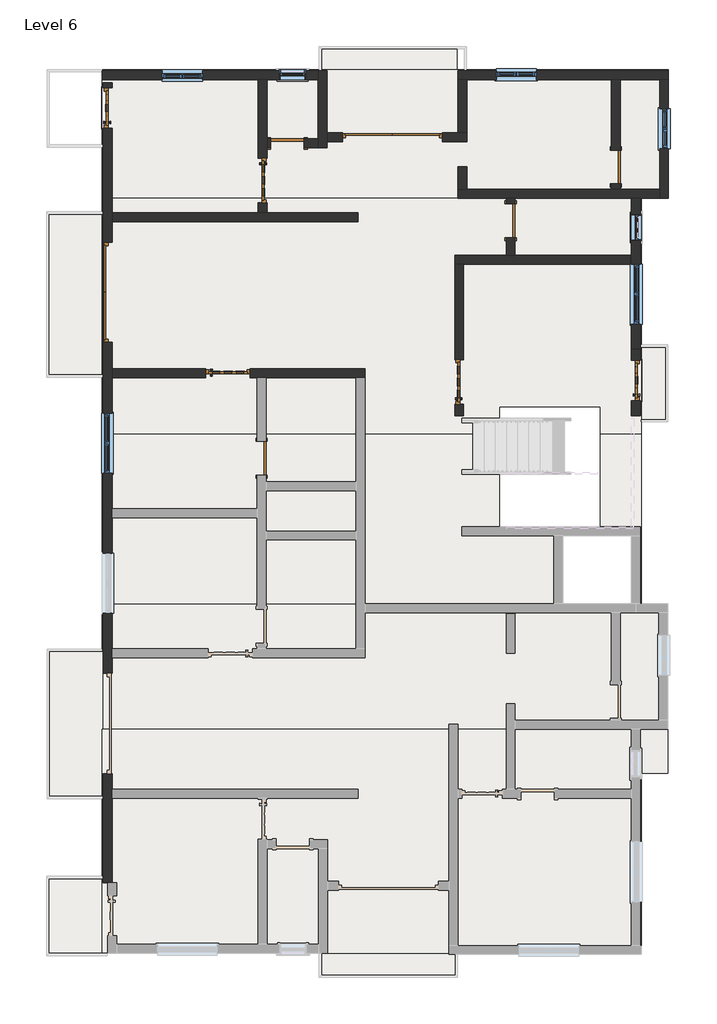
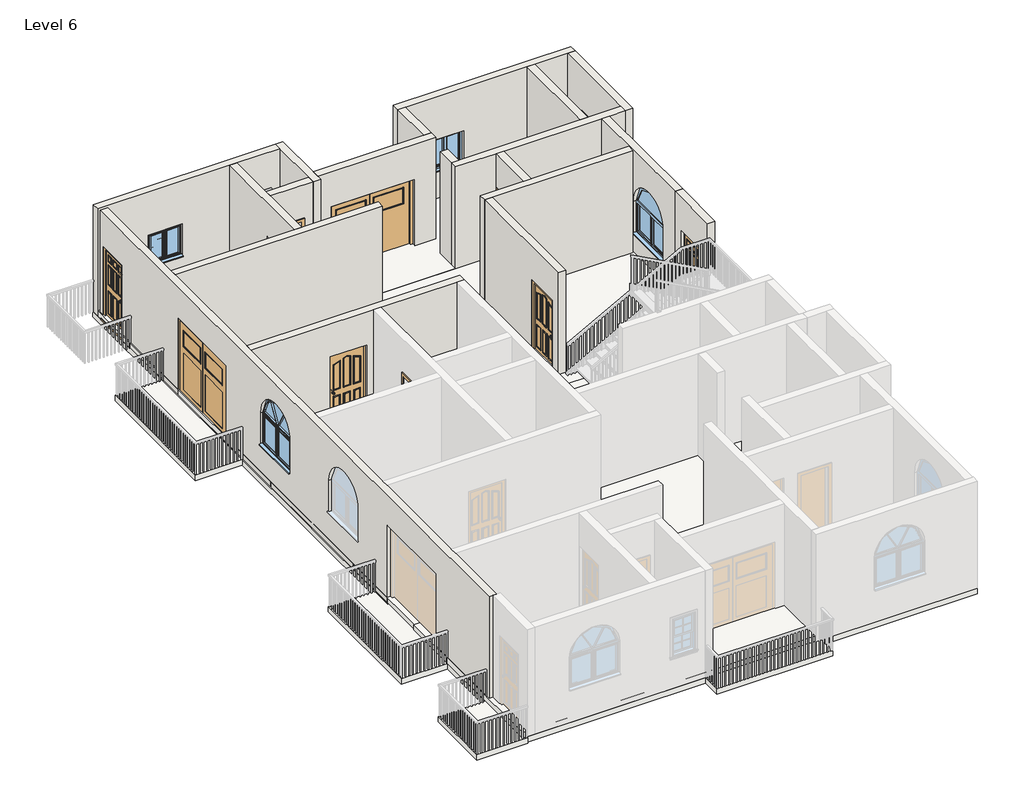
# One storey, part 2 of 7: 19 walls, 11 doors, 9 slabs, 7 windows, 5 roofs.
"""IFC4 building model written with IfcOpenShell, lengths in millimetres."""

from ifc_helpers import new_model, si_unit, point, frame, frame_2d, origin, place, context, project, spatial, polyline, circle_curve, trimmed, segment, composite_curve, outline, extrude, faceted_brep, transform, mapped, element, save
from ifc_brep_helpers import plane_surface, revolved_surface, advanced_brep
from components import doors_extsgl_5_910x2110mm_99758a98, doors_extsgl_5_910x2110mm_d3ca6061, doors_extsgl_6_1010x2110mm_b93c615f, doors_extsgl_6_1010x2110mm_efbaf1af, doors_garage_timber_side_hung_glazing_2270x2050mm_ae99176d, doors_garage_timber_side_hung_glazing_2270x2200mm_badb7014, door_53b1b562, window_679d2811, windows_arched_1360x910mm_c5754810, windows_dbl_w_glazing_bars_910x910mm_41eba874

model = new_model("IFC4")

# Units and contexts
model_context = context("Model", 3, world=origin())
ifc_project = project(units=[si_unit("LENGTHUNIT", "METRE", prefix="MILLI")], contexts=[model_context])

# Site, building, storey
site = spatial("IfcSite", under=ifc_project)
building = spatial("IfcBuilding", under=site)
storey = spatial("IfcBuildingStorey", under=building, Name="Level 6", Elevation=15240.0)

# Doors
placement = place(None, origin())
doors_extsgl_5_910x2110mm_shape = doors_extsgl_5_910x2110mm_99758a98(model_context)
element("IfcDoor", 1, ObjectType="Doors_ExtSgl_5 : 910x2110mm", at=placement, inside=storey, context=model_context, shape_type="MappedRepresentation", body=[
    mapped(doors_extsgl_5_910x2110mm_shape, transform((5761.5890963, 2376.5107951, 15240.0), x_axis=(0.0, 1.0, 0.0), y_axis=(-1.0, 0.0, 0.0), z_axis=(0.0, 0.0, 1.0))),
])
doors_extsgl_5_910x2110mm_2_shape = doors_extsgl_5_910x2110mm_d3ca6061(model_context)
element("IfcDoor", 2, ObjectType="Doors_ExtSgl_5 : 910x2110mm", at=placement, inside=storey, context=model_context, shape_type="MappedRepresentation", body=[
    mapped(doors_extsgl_5_910x2110mm_2_shape, transform((-6229.2013636, 8553.74399, 15240.0), x_axis=(0.0, 1.0, 0.0), y_axis=(-1.0, 0.0, 0.0), z_axis=(0.0, 0.0, 1.0))),
])
doors_extsgl_6_1010x2110mm_shape = doors_extsgl_6_1010x2110mm_b93c615f(model_context)
doors_extsgl_6_1010x2110mm_2_shape = doors_extsgl_6_1010x2110mm_efbaf1af(model_context)
element("IfcDoor", 3, ObjectType="Doors_ExtSgl_6 : 1010x2110mm", at=placement, inside=storey, context=model_context, shape_type="MappedRepresentation", body=[
    mapped(doors_extsgl_6_1010x2110mm_shape, transform((-2709.3109037, 6913.1295584, 15240.0), x_axis=(0.0, -1.0, 0.0), y_axis=(1.0, 0.0, 0.0), z_axis=(0.0, 0.0, 1.0))),
    mapped(doors_extsgl_6_1010x2110mm_2_shape, transform((-2709.3109037, 6913.1295584, 15240.0), x_axis=(0.0, -1.0, 0.0), y_axis=(1.0, 0.0, 0.0), z_axis=(0.0, 0.0, 1.0))),
])
element("IfcDoor", 4, ObjectType="Doors_ExtSgl_6 : 1010x2110mm", at=placement, inside=storey, context=model_context, shape_type="MappedRepresentation", body=[
    mapped(doors_extsgl_6_1010x2110mm_shape, transform((1748.3890963, 2341.0628918, 15240.0), x_axis=(0.0, 1.0, 0.0), y_axis=(-1.0, 0.0, 0.0), z_axis=(0.0, 0.0, 1.0))),
    mapped(doors_extsgl_6_1010x2110mm_2_shape, transform((1748.3890963, 2341.0628918, 15240.0), x_axis=(0.0, 1.0, 0.0), y_axis=(-1.0, 0.0, 0.0), z_axis=(0.0, 0.0, 1.0))),
])
element("IfcDoor", 5, ObjectType="Doors_ExtSgl_6 : 1010x2110mm", at=placement, inside=storey, context=model_context, shape_type="MappedRepresentation", body=[
    mapped(doors_extsgl_6_1010x2110mm_shape, transform((-3496.7442371, 2544.2962251, 15240.0), x_axis=(1.0, 0.0, 0.0), y_axis=(0.0, 1.0, 0.0), z_axis=(0.0, 0.0, 1.0))),
    mapped(doors_extsgl_6_1010x2110mm_2_shape, transform((-3496.7442371, 2544.2962251, 15240.0), x_axis=(1.0, 0.0, 0.0), y_axis=(0.0, 1.0, 0.0), z_axis=(0.0, 0.0, 1.0))),
])
doors_garage_timber_side_hung_glazing_2270x2050mm_shape = doors_garage_timber_side_hung_glazing_2270x2050mm_ae99176d(model_context)
element("IfcDoor", 6, ObjectType="Doors_Garage_Timber_Side_Hung_Glazing : 2270x2050mm", at=placement, inside=storey, context=model_context, shape_type="MappedRepresentation", body=[
    mapped(doors_garage_timber_side_hung_glazing_2270x2050mm_shape, transform((237.0890963, 7890.9962251, 15240.0), x_axis=(1.0, 0.0, 0.0), y_axis=(0.0, 1.0, 0.0), z_axis=(0.0, 0.0, 1.0))),
])
doors_garage_timber_side_hung_glazing_2270x2200mm_shape = doors_garage_timber_side_hung_glazing_2270x2200mm_badb7014(model_context)
element("IfcDoor", 7, ObjectType="Doors_Garage_Timber_Side_Hung_Glazing : 2270x2200mm", at=placement, inside=storey, context=model_context, shape_type="MappedRepresentation", body=[
    mapped(doors_garage_timber_side_hung_glazing_2270x2200mm_shape, transform((-6229.2013636, 4373.0962251, 15240.0), x_axis=(0.0, -1.0, 0.0), y_axis=(1.0, 0.0, 0.0), z_axis=(0.0, 0.0, 1.0))),
])
door_shape = door_53b1b562(model_context)
element("IfcDoor", 8, ObjectType="Single-Flush : 30\" x 80\"", at=placement, inside=storey, context=model_context, shape_type="MappedRepresentation", body=[
    mapped(door_shape, transform((-2150.5109037, 7751.2962251, 15240.0), x_axis=(-1.0, 0.0, 0.0), y_axis=(0.0, -1.0, 0.0), z_axis=(0.0, 0.0, 1.0))),
])
element("IfcDoor", 9, ObjectType="Single-Flush : 30\" x 80\"", at=placement, inside=storey, context=model_context, shape_type="MappedRepresentation", body=[
    mapped(door_shape, transform((2916.7890963, 5998.6962251, 15240.0), x_axis=(0.0, 1.0, 0.0), y_axis=(-1.0, 0.0, 0.0), z_axis=(0.0, 0.0, 1.0))),
])
element("IfcDoor", 10, ObjectType="Single-Flush : 30\" x 80\"", at=placement, inside=storey, context=model_context, shape_type="MappedRepresentation", body=[
    mapped(door_shape, transform((-2734.7109037, 613.8962251, 15240.0), x_axis=(0.0, 1.0, 0.0), y_axis=(-1.0, 0.0, 0.0), z_axis=(0.0, 0.0, 1.0))),
])
element("IfcDoor", 11, ObjectType="Single-Flush : 30\" x 80\"", at=placement, inside=storey, context=model_context, shape_type="MappedRepresentation", body=[
    mapped(door_shape, transform((5304.3890963, 7217.8962251, 15240.0), x_axis=(0.0, 1.0, 0.0), y_axis=(-1.0, 0.0, 0.0), z_axis=(0.0, 0.0, 1.0))),
])

# Roofs
element("IfcRoof", 12, ObjectType="Generic - 12\"", at=placement, inside=storey, context=model_context, shape_type="SweptSolid", body=[
    extrude(outline(polyline([(-6354.2109037, 9427.2527313), (6498.1890963, 9427.2527313), (6498.1890963, 6506.6962251), (-6354.2109037, 6506.6962251), (-6354.2109037, 9427.2527313)])), frame((0.0, 0.0, 15240.0), z_axis=(0.0, 0.0, 1.0), x_axis=(1.0, 0.0, 0.0)), (0.0, 0.0, 1.0), 152.4),
])
element("IfcRoof", 13, ObjectType="Generic - 12\"", at=placement, inside=storey, context=model_context, shape_type="SweptSolid", body=[
    extrude(outline(polyline([(-6330.8013636, -2688.1037749), (6485.4890963, -2688.1037749), (6485.4890963, -6529.1251987), (-6330.8013636, -6529.1251987), (-6330.8013636, -2688.1037749)])), frame((0.0, 0.0, 15240.0), z_axis=(0.0, 0.0, 1.0), x_axis=(1.0, 0.0, 0.0)), (0.0, 0.0, 1.0), 152.4),
])
element("IfcRoof", 14, ObjectType="Generic - 12\"", at=placement, inside=storey, context=model_context, shape_type="SweptSolid", body=[
    extrude(outline(polyline([(-6354.2109037, -5532.9037749), (5863.1890963, -5532.9037749), (5863.1890963, -10612.9037749), (-6354.2109037, -10612.9037749), (-6354.2109037, -5532.9037749)])), frame((0.0, 0.0, 15240.0), z_axis=(0.0, 0.0, 1.0), x_axis=(1.0, 0.0, 0.0)), (0.0, 0.0, 1.0), 152.4),
])
element("IfcRoof", 15, ObjectType="Generic - 12\"", at=placement, inside=storey, context=model_context, shape_type="SweptSolid", body=[
    extrude(outline(polyline([(-6330.8013636, 1160.801054), (-6330.8013636, 6506.6962251), (5875.8890963, 6506.6962251), (5875.8890963, 1160.801054), (4949.8616623, 1160.801054), (4949.8616623, 1784.6684315), (2663.8616623, 1784.6684315), (2663.8616623, 1160.801054), (-6330.8013636, 1160.801054)])), frame((0.0, 0.0, 15240.0), z_axis=(0.0, 0.0, 1.0), x_axis=(1.0, 0.0, 0.0)), (0.0, 0.0, 1.0), 152.4),
])
element("IfcRoof", 16, ObjectType="Generic - 12\"", at=placement, inside=storey, context=model_context, shape_type="SweptSolid", body=[
    extrude(outline(polyline([(-6330.8013636, -2688.1037749), (-6330.8013636, 1160.801054), (2663.8616623, 1160.801054), (2663.8616623, -958.5315685), (4949.8616623, -958.5315685), (4949.8616623, 1160.801054), (5875.8890963, 1160.801054), (5875.8890963, -2688.1037749), (5659.9890963, -2688.1037749), (5659.9890963, -1138.7037749), (4097.8890963, -1138.7037749), (4097.8890963, -2688.1037749), (-6330.8013636, -2688.1037749)])), frame((0.0, 0.0, 15240.0), z_axis=(0.0, 0.0, 1.0), x_axis=(1.0, 0.0, 0.0)), (0.0, 0.0, 1.0), 152.4),
])

# Slabs
element("IfcSlab", 17, ObjectType="Generic - 12\"", at=placement, inside=storey, context=model_context, shape_type="SweptSolid", body=[
    extrude(outline(polyline([(1694.4140963, 9948.3962251), (1694.4140963, -11133.6037749), (-1426.6109037, -11133.6037749), (-1426.6109037, 9948.3962251), (1694.4140963, 9948.3962251)])), frame((0.0, 0.0, 15087.6), z_axis=(0.0, 0.0, 1.0), x_axis=(1.0, 0.0, 0.0)), (0.0, 0.0, 1.0), 152.4),
])
element("IfcSlab", 18, ObjectType="Generic - 12\"", at=placement, inside=storey, context=model_context, shape_type="SweptSolid", body=[
    extrude(outline(polyline([(5875.8890963, 9402.2962251), (5875.8890963, -10638.3037749), (1722.9890963, -10638.3037749), (1722.9890963, 9402.2962251), (5875.8890963, 9402.2962251)]), holes=[polyline([(4949.8616623, 1784.6684315), (2663.8616623, 1784.6684315), (2663.8616623, -958.5315685), (4949.8616623, -958.5315685), (4949.8616623, 1784.6684315)]), polyline([(5659.9890963, -1138.7037749), (4097.8890963, -1138.7037749), (4097.8890963, -2688.1037749), (5659.9890963, -2688.1037749), (5659.9890963, -1138.7037749)])]), frame((0.0, 0.0, 15087.6), z_axis=(0.0, 0.0, 1.0), x_axis=(1.0, 0.0, 0.0)), (0.0, 0.0, 1.0), 152.4),
])
element("IfcSlab", 19, ObjectType="Generic - 12\"", at=placement, inside=storey, context=model_context, shape_type="SweptSolid", body=[
    extrude(outline(polyline([(6498.1890963, 9402.2962251), (6498.1890963, 6506.6962251), (5875.8890963, 6506.6962251), (5875.8890963, 9402.2962251), (6498.1890963, 9402.2962251)])), frame((0.0, 0.0, 15087.6), z_axis=(0.0, 0.0, 1.0), x_axis=(1.0, 0.0, 0.0)), (0.0, 0.0, 1.0), 152.4),
])
element("IfcSlab", 20, ObjectType="Generic - 12\"", at=placement, inside=storey, context=model_context, shape_type="SweptSolid", body=[
    extrude(outline(polyline([(6485.4890963, 3183.81308), (6485.4890963, 1439.3962251), (5863.1890963, 1439.3962251), (5863.1890963, 3183.81308), (6485.4890963, 3183.81308)])), frame((0.0, 0.0, 15087.6), z_axis=(0.0, 0.0, 1.0), x_axis=(1.0, 0.0, 0.0)), (0.0, 0.0, 1.0), 152.4),
])
element("IfcSlab", 21, ObjectType="Generic - 12\"", at=placement, inside=storey, context=model_context, shape_type="SweptSolid", body=[
    extrude(outline(polyline([(6485.4890963, -2688.1037749), (6485.4890963, -5532.9037749), (5863.1890963, -5532.9037749), (5863.1890963, -2688.1037749), (6485.4890963, -2688.1037749)])), frame((0.0, 0.0, 15087.6), z_axis=(0.0, 0.0, 1.0), x_axis=(1.0, 0.0, 0.0)), (0.0, 0.0, 1.0), 152.4),
])
element("IfcSlab", 22, ObjectType="Generic - 12\"", at=placement, inside=storey, context=model_context, shape_type="SweptSolid", body=[
    extrude(outline(polyline([(-6330.8013636, 6201.8962251), (-6330.8013636, 2455.3962251), (-7614.6859037, 2455.3962251), (-7614.6859037, 6201.8962251), (-6330.8013636, 6201.8962251)])), frame((0.0, 0.0, 15087.6), z_axis=(0.0, 0.0, 1.0), x_axis=(1.0, 0.0, 0.0)), (0.0, 0.0, 1.0), 152.4),
])
element("IfcSlab", 23, ObjectType="Generic - 12\"", at=placement, inside=storey, context=model_context, shape_type="SweptSolid", body=[
    extrude(outline(polyline([(-6330.8013636, -3716.8037749), (-6330.8013636, -7105.2894702), (-7598.8109037, -7105.2894702), (-7598.8109037, -3716.8037749), (-6330.8013636, -3716.8037749)])), frame((0.0, 0.0, 15087.6), z_axis=(0.0, 0.0, 1.0), x_axis=(1.0, 0.0, 0.0)), (0.0, 0.0, 1.0), 152.4),
])
element("IfcSlab", 24, ObjectType="Generic - 12\"", at=placement, inside=storey, context=model_context, shape_type="SweptSolid", body=[
    extrude(outline(polyline([(-6243.0859037, -8868.0845215), (-6243.0859037, -10663.7037749), (-7614.6859037, -10663.7037749), (-7614.6859037, -8868.0845215), (-6243.0859037, -8868.0845215)])), frame((0.0, 0.0, 15087.6), z_axis=(0.0, 0.0, 1.0), x_axis=(1.0, 0.0, 0.0)), (0.0, 0.0, 1.0), 152.4),
])
element("IfcSlab", 25, ObjectType="Generic - 12\"", at=placement, inside=storey, context=model_context, shape_type="SweptSolid", body=[
    extrude(outline(polyline([(-1236.1109037, 9427.2527313), (-1236.1109037, -10612.9037749), (-6354.2109037, -10612.9037749), (-6354.2109037, 9427.2527313), (-1236.1109037, 9427.2527313)])), frame((0.0, 0.0, 15087.6), z_axis=(0.0, 0.0, 1.0), x_axis=(1.0, 0.0, 0.0)), (0.0, 0.0, 1.0), 152.4),
])

# Walls
element("IfcWall", 26, ObjectType="Generic - 9\" w", at=placement, inside=storey, context=model_context, shape_type="Brep", body=[
    faceted_brep([(1722.9890963, 9199.0962251, 15240.0), (1926.1890963, 9199.0962251, 15240.0), (5202.7890963, 9199.0962251, 15240.0), (5405.9890963, 9199.0962251, 15240.0), (6294.9890963, 9199.0962251, 15240.0), (6498.1890963, 9199.0962251, 15240.0), (6498.1890963, 9199.0962251, 18288.0), (6294.9890963, 9199.0962251, 18288.0), (5405.9890963, 9199.0962251, 18288.0), (5202.7890963, 9199.0962251, 18288.0), (1926.1890963, 9199.0962251, 18288.0), (1722.9890963, 9199.0962251, 18288.0), (2588.7890963, 9199.0962251, 17064.4), (3498.7890963, 9199.0962251, 17064.4), (3498.7890963, 9199.0962251, 16154.4), (2588.7890963, 9199.0962251, 16154.4), (1722.9890963, 9402.2962251, 15240.0), (1722.9890963, 9402.2962251, 18288.0), (6498.1890963, 9402.2962251, 18288.0), (6498.1890963, 9402.2962251, 15240.0), (2588.7890963, 9402.2962251, 17064.4), (2588.7890963, 9402.2962251, 16154.4), (3498.7890963, 9402.2962251, 16154.4), (3498.7890963, 9402.2962251, 17064.4)], [[[0, 1, 2, 3, 4, 5, 6, 7, 8, 9, 10, 11], [12, 13, 14, 15]], [[16, 17, 18, 19], [20, 21, 22, 23]], [[5, 4, 3, 2, 1, 0, 16, 19]], [[11, 10, 9, 8, 7, 6, 18, 17]], [[0, 11, 17, 16]], [[6, 5, 19, 18]], [[21, 20, 12, 15]], [[22, 21, 15, 14]], [[23, 22, 14, 13]], [[20, 23, 13, 12]]]),
])
element("IfcWall", 27, ObjectType="Generic - 9\" w", at=placement, inside=storey, context=model_context, shape_type="SweptSolid", body=[
    extrude(outline(polyline([(6506.6962251, 15240.0), (3087.7441284, 15240.0), (3087.7441284, 18288.0), (6506.6962251, 18288.0), (6506.6962251, 15240.0)]), holes=[polyline([(6151.0962251, 17221.2), (5541.4962251, 17221.2), (5541.4962251, 16154.4), (6151.0962251, 16154.4), (6151.0962251, 17221.2)]), composite_curve([segment(polyline([(5016.7786331, 15925.6617803), (5016.7786331, 16835.6617803)]), True, "CONTINUOUS"), segment(trimmed(circle_curve(frame_2d((4336.7786331, 16835.6617803)), 680.0), [point((5016.7786331, 16835.6617803))], [point((3656.7786331, 16835.6617803))], True, "CARTESIAN"), True, "CONTINUOUS"), segment(polyline([(3656.7786331, 16835.6617803), (3656.7786331, 15925.6617803), (5016.7786331, 15925.6617803)]), True, "CONTINUOUS")], self_intersect=False)]), frame((5659.9890963, 0.0, 0.0), z_axis=(1.0, 0.0, 0.0), x_axis=(0.0, 1.0, 0.0)), (0.0, 0.0, 1.0), 203.2),
])
element("IfcWall", 28, ObjectType="Generic - 9\" w", at=placement, inside=storey, context=model_context, shape_type="AdvancedBrep", body=[
    advanced_brep(
    [(-6330.8013636, 3238.0962251, 15240.0), (-6330.8013636, -4267.1251987, 15240.0), (-6330.8013636, -4267.1251987, 17440.0), (-6330.8013636, -6537.1251987, 17440.0), (-6330.8013636, -6537.1251987, 15240.0), (-6330.8013636, -9007.7845215, 15240.0), (-6330.8013636, -9007.7845215, 18288.0), (-6330.8013636, 9129.8816143, 18288.0), (-6330.8013636, 9129.8816143, 15240.0), (-6330.8013636, 9008.7773233, 15240.0), (-6330.8013636, 9008.7773233, 17350.0), (-6330.8013636, 8098.7773233, 17350.0), (-6330.8013636, 8098.7773233, 15240.0), (-6330.8013636, 5508.0962251, 15240.0), (-6330.8013636, 5508.0962251, 17440.0), (-6330.8013636, 3238.0962251, 17440.0), (-6330.8013636, 276.7962251, 16154.4), (-6330.8013636, 1636.7962251, 16154.4), (-6330.8013636, 1636.7962251, 17064.4), (-6330.8013636, 276.7962251, 17064.4), (-6330.8013636, -1538.2037749, 16154.4), (-6330.8013636, -1538.2037749, 17064.4), (-6330.8013636, -2898.2037749, 17064.4), (-6330.8013636, -2898.2037749, 16154.4), (-6127.6013636, -4267.1251987, 17440.0), (-6127.6013636, -4267.1251987, 15240.0), (-6127.6013636, -3907.3037749, 15240.0), (-6127.6013636, -3704.1037749, 15240.0), (-6127.6013636, -732.3037749, 15240.0), (-6127.6013636, -529.1037749, 15240.0), (-6127.6013636, 2442.6962251, 15240.0), (-6127.6013636, 2645.8962251, 15240.0), (-6127.6013636, 3238.0962251, 15240.0), (-6127.6013636, 3238.0962251, 17440.0), (-6127.6013636, 5508.0962251, 17440.0), (-6127.6013636, 5508.0962251, 15240.0), (-6127.6013636, 5973.2962251, 15240.0), (-6127.6013636, 6176.4962251, 15240.0), (-6127.6013636, 8098.7773233, 15240.0), (-6127.6013636, 8098.7773233, 17350.0), (-6127.6013636, 9008.7773233, 17350.0), (-6127.6013636, 9008.7773233, 15240.0), (-6127.6013636, 9129.8816143, 15240.0), (-6127.6013636, 9129.8816143, 18288.0), (-6127.6013636, 6176.4962251, 18288.0), (-6127.6013636, 5973.2962251, 18288.0), (-6127.6013636, 2645.8962251, 18288.0), (-6127.6013636, 2442.6962251, 18288.0), (-6127.6013636, -529.1037749, 18288.0), (-6127.6013636, -732.3037749, 18288.0), (-6127.6013636, -3704.1037749, 18288.0), (-6127.6013636, -3907.3037749, 18288.0), (-6127.6013636, -6896.9466225, 18288.0), (-6127.6013636, -7100.1466225, 18288.0), (-6127.6013636, -9007.7845215, 18288.0), (-6127.6013636, -9007.7845215, 15240.0), (-6127.6013636, -7100.1466225, 15240.0), (-6127.6013636, -6896.9466225, 15240.0), (-6127.6013636, -6537.1251987, 15240.0), (-6127.6013636, -6537.1251987, 17440.0), (-6127.6013636, 276.7962251, 16154.4), (-6127.6013636, 276.7962251, 17064.4), (-6127.6013636, 1636.7962251, 17064.4), (-6127.6013636, 1636.7962251, 16154.4), (-6127.6013636, -1538.2037749, 16154.4), (-6127.6013636, -2898.2037749, 16154.4), (-6127.6013636, -2898.2037749, 17064.4), (-6127.6013636, -1538.2037749, 17064.4), (-6229.2013636, -9007.7845215, 15240.0), (-6229.2013636, -9007.7845215, 18288.0)],
    [
        (0, 1),
        (1, 2),
        (2, 3),
        (3, 4),
        (4, 5),
        (5, 6),
        (6, 7),
        (7, 8),
        (8, 9),
        (9, 10),
        (10, 11),
        (11, 12),
        (12, 13),
        (13, 14),
        (14, 15),
        (15, 0),
        (16, 17),
        (17, 18),
        (18, 19, circle_curve(frame((-6330.8013636, 956.7962251, 17064.4), z_axis=(1.0, 0.0, 0.0), x_axis=(0.0, 1.0, 0.0)), 680.0)),
        (19, 16),
        (20, 21),
        (21, 22, circle_curve(frame((-6330.8013636, -2218.2037749, 17064.4), z_axis=(1.0, 0.0, 0.0), x_axis=(0.0, -1.0, 0.0)), 680.0)),
        (22, 23),
        (23, 20),
        (24, 25),
        (25, 26),
        (26, 27),
        (27, 28),
        (28, 29),
        (29, 30),
        (30, 31),
        (31, 32),
        (32, 33),
        (33, 34),
        (34, 35),
        (35, 36),
        (36, 37),
        (37, 38),
        (38, 39),
        (39, 40),
        (40, 41),
        (41, 42),
        (42, 43),
        (43, 44),
        (44, 45),
        (45, 46),
        (46, 47),
        (47, 48),
        (48, 49),
        (49, 50),
        (50, 51),
        (51, 52),
        (52, 53),
        (53, 54),
        (54, 55),
        (55, 56),
        (56, 57),
        (57, 58),
        (58, 59),
        (59, 24),
        (60, 61),
        (61, 62, circle_curve(frame((-6127.6013636, 956.7962251, 17064.4), z_axis=(-1.0, 0.0, 0.0), x_axis=(0.0, 1.0, 0.0)), 680.0)),
        (62, 63),
        (63, 60),
        (64, 65),
        (65, 66),
        (66, 67, circle_curve(frame((-6127.6013636, -2218.2037749, 17064.4), z_axis=(-1.0, 0.0, 0.0), x_axis=(0.0, -1.0, 0.0)), 680.0)),
        (67, 64),
        (41, 9),
        (8, 42),
        (12, 38),
        (35, 13),
        (55, 68),
        (68, 5),
        (4, 58),
        (25, 1),
        (0, 32),
        (54, 69),
        (69, 6),
        (43, 7),
        (11, 39),
        (40, 10),
        (34, 14),
        (15, 33),
        (3, 59),
        (24, 2),
        (60, 16),
        (19, 61),
        (18, 62),
        (17, 63),
        (20, 64),
        (67, 21),
        (66, 22),
        (65, 23),
    ],
    [
        plane_surface(frame((-6330.8013636, 2442.6962251, 15240.0), z_axis=(-1.0, 0.0, 0.0), x_axis=(0.0, -1.0, 0.0))),
        plane_surface(frame((-6127.6013636, 2442.6962251, 15240.0), z_axis=(1.0, 0.0, 0.0), x_axis=(0.0, 1.0, 0.0))),
        plane_surface(frame((-6330.8013636, 9129.8816143, 15240.0), z_axis=(0.0, 0.0, -1.0), x_axis=(1.0, 0.0, 0.0))),
        plane_surface(frame((-6330.8013636, -9007.7845215, 15240.0), z_axis=(0.0, -1.0, 0.0), x_axis=(1.0, 0.0, 0.0))),
        plane_surface(frame((-6330.8013636, -9007.7845215, 18288.0), z_axis=(0.0, 0.0, 1.0), x_axis=(1.0, 0.0, 0.0))),
        plane_surface(frame((-6330.8013636, 9129.8816143, 18288.0), z_axis=(0.0, 1.0, 0.0), x_axis=(1.0, 0.0, 0.0))),
        plane_surface(frame((-6330.8013636, 8098.7773233, 17350.0), z_axis=(0.0, 1.0, 0.0), x_axis=(1.0, 0.0, 0.0))),
        plane_surface(frame((-6330.8013636, 9008.7773233, 15240.0), z_axis=(0.0, -1.0, 0.0), x_axis=(1.0, 0.0, 0.0))),
        plane_surface(frame((-6330.8013636, 9008.7773233, 17350.0), z_axis=(0.0, 0.0, -1.0), x_axis=(1.0, 0.0, 0.0))),
        plane_surface(frame((-6127.6013636, 5508.0962251, 17440.0), z_axis=(0.0, -1.0, 0.0), x_axis=(-1.0, 0.0, 0.0))),
        plane_surface(frame((-6127.6013636, 3238.0962251, 15240.0), z_axis=(0.0, 1.0, 0.0), x_axis=(-1.0, 0.0, 0.0))),
        plane_surface(frame((-6127.6013636, 3238.0962251, 17440.0), z_axis=(0.0, 0.0, -1.0), x_axis=(-1.0, 0.0, 0.0))),
        plane_surface(frame((-6330.8013636, -6537.1251987, 17440.0), z_axis=(0.0, 1.0, 0.0), x_axis=(1.0, 0.0, 0.0))),
        plane_surface(frame((-6330.8013636, -4267.1251987, 15240.0), z_axis=(0.0, -1.0, 0.0), x_axis=(1.0, 0.0, 0.0))),
        plane_surface(frame((-6330.8013636, -4267.1251987, 17440.0), z_axis=(0.0, 0.0, -1.0), x_axis=(1.0, 0.0, 0.0))),
        plane_surface(frame((-6127.6013636, 276.7962251, 16154.4), z_axis=(0.0, 1.0, 0.0), x_axis=(-1.0, 0.0, 0.0))),
        revolved_surface(polyline([(-6330.8013636, 1636.7962251, 17064.4), (-6127.6013636, 1636.7962251, 17064.4)]), (-6127.6013636, 956.7962251, 17064.4), (-1.0, 0.0, 0.0)),
        plane_surface(frame((-6127.6013636, 1636.7962251, 17064.4), z_axis=(0.0, -1.0, 0.0), x_axis=(-1.0, 0.0, 0.0))),
        plane_surface(frame((-6127.6013636, 1636.7962251, 16154.4), z_axis=(0.0, 0.0, 1.0), x_axis=(-1.0, 0.0, 0.0))),
        plane_surface(frame((-6330.8013636, -1538.2037749, 16154.4), z_axis=(0.0, -1.0, 0.0), x_axis=(1.0, 0.0, 0.0))),
        revolved_surface(polyline([(-6127.6013636, -2898.2037749, 17064.4), (-6330.8013636, -2898.2037749, 17064.4)]), (-6330.8013636, -2218.2037749, 17064.4), (1.0, 0.0, 0.0)),
        plane_surface(frame((-6330.8013636, -2898.2037749, 17064.4), z_axis=(0.0, 1.0, 0.0), x_axis=(1.0, 0.0, 0.0))),
        plane_surface(frame((-6330.8013636, -2898.2037749, 16154.4), z_axis=(0.0, 0.0, 1.0), x_axis=(1.0, 0.0, 0.0))),
    ],
    [
        (0, [[1, 2, 3, 4, 5, 6, 7, 8, 9, 10, 11, 12, 13, 14, 15, 16], [17, 18, 19, 20], [21, 22, 23, 24]]),
        (1, [[25, 26, 27, 28, 29, 30, 31, 32, 33, 34, 35, 36, 37, 38, 39, 40, 41, 42, 43, 44, 45, 46, 47, 48, 49, 50, 51, 52, 53, 54, 55, 56, 57, 58, 59, 60], [61, 62, 63, 64], [65, 66, 67, 68]]),
        (2, [[-42, 69, -9, 70]]),
        (2, [[-13, 71, -38, -37, -36, 72]]),
        (2, [[-58, -57, -56, 73, 74, -5, 75]]),
        (2, [[-32, -31, -30, -29, -28, -27, -26, 76, -1, 77]]),
        (3, [[-6, -74, -73, -55, 78, 79]]),
        (4, [[-7, -79, -78, -54, -53, -52, -51, -50, -49, -48, -47, -46, -45, -44, 80]]),
        (5, [[-8, -80, -43, -70]]),
        (6, [[-12, 81, -39, -71]]),
        (7, [[-10, -69, -41, 82]]),
        (8, [[-11, -82, -40, -81]]),
        (9, [[-35, 83, -14, -72]]),
        (10, [[-33, -77, -16, 84]]),
        (11, [[-34, -84, -15, -83]]),
        (12, [[-4, 85, -59, -75]]),
        (13, [[-2, -76, -25, 86]]),
        (14, [[-3, -86, -60, -85]]),
        (15, [[-61, 87, -20, 88]]),
        (16, [[-62, -88, -19, 89]]),
        (17, [[-63, -89, -18, 90]]),
        (18, [[-64, -90, -17, -87]]),
        (19, [[-21, 91, -68, 92]]),
        (20, [[-22, -92, -67, 93]]),
        (21, [[-23, -93, -66, 94]]),
        (22, [[-24, -94, -65, -91]]),
    ],
),
])
element("IfcWall", 29, ObjectType="Generic - 9\" w", at=placement, inside=storey, context=model_context, shape_type="SweptSolid", body=[
    extrude(outline(polyline([(3087.7441284, 15240.0), (2831.5441284, 15240.0), (2831.5441284, 17350.0), (1921.5441284, 17350.0), (1921.5441284, 15240.0), (1579.0962251, 15240.0), (1579.0962251, 18288.0), (3087.7441284, 18288.0), (3087.7441284, 15240.0)])), frame((5659.9890963, 0.0, 0.0), z_axis=(1.0, 0.0, 0.0), x_axis=(0.0, 1.0, 0.0)), (0.0, 0.0, 1.0), 203.2),
])
element("IfcWall", 30, ObjectType="Generic - 9\" w", at=placement, inside=storey, context=model_context, shape_type="Brep", body=[
    faceted_brep([(-1452.0109037, 9401.8527313, 15240.0), (-6354.2109037, 9401.8527313, 15240.0), (-6354.2109037, 9401.8527313, 18288.0), (-1452.0109037, 9401.8527313, 18288.0), (-4076.7609037, 9401.8527313, 17064.4), (-4986.7609037, 9401.8527313, 17064.4), (-4986.7609037, 9401.8527313, 16154.4), (-4076.7609037, 9401.8527313, 16154.4), (-2334.6609037, 9401.8527313, 17221.2), (-2334.6609037, 9401.8527313, 16154.4), (-1725.0609037, 9401.8527313, 16154.4), (-1725.0609037, 9401.8527313, 17221.2), (-1452.0109037, 9198.6527313, 15240.0), (-1452.0109037, 9198.6527313, 18288.0), (-2607.7109037, 9198.6527313, 18288.0), (-2810.9109037, 9198.6527313, 18288.0), (-6354.2109037, 9198.6527313, 18288.0), (-6354.2109037, 9198.6527313, 15240.0), (-2810.9109037, 9198.6527313, 15240.0), (-2607.7109037, 9198.6527313, 15240.0), (-4076.7609037, 9198.6527313, 17064.4), (-4076.7609037, 9198.6527313, 16154.4), (-4986.7609037, 9198.6527313, 16154.4), (-4986.7609037, 9198.6527313, 17064.4), (-2334.6609037, 9198.6527313, 17221.2), (-1725.0609037, 9198.6527313, 17221.2), (-1725.0609037, 9198.6527313, 16154.4), (-2334.6609037, 9198.6527313, 16154.4)], [[[0, 1, 2, 3], [4, 5, 6, 7], [8, 9, 10, 11]], [[12, 13, 14, 15, 16, 17, 18, 19], [20, 21, 22, 23], [24, 25, 26, 27]], [[1, 0, 12, 19, 18, 17]], [[2, 1, 17, 16]], [[3, 2, 16, 15, 14, 13]], [[0, 3, 13, 12]], [[21, 20, 4, 7]], [[22, 21, 7, 6]], [[23, 22, 6, 5]], [[20, 23, 5, 4]], [[9, 8, 24, 27]], [[10, 9, 27, 26]], [[11, 10, 26, 25]], [[8, 11, 25, 24]]]),
])
element("IfcWall", 31, ObjectType="Generic -4.5\" p", at=placement, inside=storey, context=model_context, shape_type="Brep", body=[
    faceted_brep([(-2810.9109037, 6408.0962251, 17350.0), (-2810.9109037, 6408.0962251, 15240.0), (-2810.9109037, 6176.4962251, 15240.0), (-2810.9109037, 6176.4962251, 18288.0), (-2810.9109037, 9198.6527313, 18288.0), (-2810.9109037, 9198.6527313, 15240.0), (-2810.9109037, 7418.0962251, 15240.0), (-2810.9109037, 7418.0962251, 17350.0), (-2607.7109037, 6176.4962251, 15240.0), (-2607.7109037, 6408.0962251, 15240.0), (-2607.7109037, 6408.0962251, 17350.0), (-2607.7109037, 7418.0962251, 17350.0), (-2607.7109037, 7418.0962251, 15240.0), (-2607.7109037, 7649.6962251, 15240.0), (-2607.7109037, 7852.8962251, 15240.0), (-2607.7109037, 9198.6527313, 15240.0), (-2607.7109037, 9198.6527313, 18288.0), (-2607.7109037, 7852.8962251, 18288.0), (-2607.7109037, 7649.6962251, 18288.0), (-2607.7109037, 6176.4962251, 18288.0)], [[[0, 1, 2, 3, 4, 5, 6, 7]], [[8, 9, 10, 11, 12, 13, 14, 15, 16, 17, 18, 19]], [[6, 5, 15, 14, 13, 12]], [[2, 1, 9, 8]], [[4, 3, 19, 18, 17, 16]], [[3, 2, 8, 19]], [[12, 11, 7, 6]], [[10, 9, 1, 0]], [[11, 10, 0, 7]], [[5, 4, 16, 15]]]),
])
element("IfcWall", 32, ObjectType="Generic -4.5\" p", at=placement, inside=storey, context=model_context, shape_type="Brep", body=[
    faceted_brep([(-6127.6013636, 5973.2962251, 15240.0), (-550.3109037, 5973.2962251, 15240.0), (-550.3109037, 5973.2962251, 18288.0), (-6127.6013636, 5973.2962251, 18288.0), (-6127.6013636, 6176.4962251, 15240.0), (-6127.6013636, 6176.4962251, 18288.0), (-2810.9109037, 6176.4962251, 18288.0), (-2607.7109037, 6176.4962251, 18288.0), (-550.3109037, 6176.4962251, 18288.0), (-550.3109037, 6176.4962251, 15240.0), (-2607.7109037, 6176.4962251, 15240.0), (-2810.9109037, 6176.4962251, 15240.0)], [[[0, 1, 2, 3]], [[4, 5, 6, 7, 8, 9, 10, 11]], [[1, 0, 4, 11, 10, 9]], [[2, 1, 9, 8]], [[3, 2, 8, 7, 6, 5]], [[0, 3, 5, 4]]]),
])
element("IfcWall", 33, ObjectType="Generic -4.5\" p", at=placement, inside=storey, context=model_context, shape_type="Brep", body=[
    faceted_brep([(-1452.0109037, 9401.8527313, 15240.0), (-1452.0109037, 9198.6527313, 15240.0), (-1452.0109037, 7852.8962251, 15240.0), (-1452.0109037, 7649.6962251, 15240.0), (-1452.0109037, 7649.6962251, 18288.0), (-1452.0109037, 7852.8962251, 18288.0), (-1452.0109037, 9198.6527313, 18288.0), (-1452.0109037, 9401.8527313, 18288.0), (-1248.8109037, 9401.8527313, 15240.0), (-1248.8109037, 9401.8527313, 18288.0), (-1248.8109037, 7992.5962251, 18288.0), (-1248.8109037, 7789.3962251, 18288.0), (-1248.8109037, 7649.6962251, 18288.0), (-1248.8109037, 7649.6962251, 15240.0), (-1248.8109037, 7789.3962251, 15240.0), (-1248.8109037, 7992.5962251, 15240.0)], [[[0, 1, 2, 3, 4, 5, 6, 7]], [[8, 9, 10, 11, 12, 13, 14, 15]], [[3, 2, 1, 0, 8, 15, 14, 13]], [[7, 6, 5, 4, 12, 11, 10, 9]], [[4, 3, 13, 12]], [[0, 7, 9, 8]]]),
])
element("IfcWall", 34, ObjectType="Generic -4.5\" p", at=placement, inside=storey, context=model_context, shape_type="SweptSolid", body=[
    extrude(outline(polyline([(15240.0, -2607.7109037), (15240.0, -2531.5109037), (17272.0, -2531.5109037), (17272.0, -1769.5109037), (15240.0, -1769.5109037), (15240.0, -1452.0109037), (18288.0, -1452.0109037), (18288.0, -2607.7109037), (15240.0, -2607.7109037)])), frame((0.0, 7649.6962251, 0.0), z_axis=(0.0, 1.0, 0.0), x_axis=(0.0, 0.0, 1.0)), (0.0, 0.0, 1.0), 203.2),
])
element("IfcWall", 35, ObjectType="Generic -4.5\" p", at=placement, inside=storey, context=model_context, shape_type="Brep", body=[
    faceted_brep([(1372.0890963, 7789.3962251, 17290.0), (1372.0890963, 7789.3962251, 15240.0), (1926.1890963, 7789.3962251, 15240.0), (1926.1890963, 7789.3962251, 18288.0), (-1248.8109037, 7789.3962251, 18288.0), (-1248.8109037, 7789.3962251, 15240.0), (-897.9109037, 7789.3962251, 15240.0), (-897.9109037, 7789.3962251, 17290.0), (1926.1890963, 7992.5962251, 15240.0), (1722.9890963, 7992.5962251, 15240.0), (1372.0890963, 7992.5962251, 15240.0), (1372.0890963, 7992.5962251, 17290.0), (-897.9109037, 7992.5962251, 17290.0), (-897.9109037, 7992.5962251, 15240.0), (-1248.8109037, 7992.5962251, 15240.0), (-1248.8109037, 7992.5962251, 18288.0), (1722.9890963, 7992.5962251, 18288.0), (1926.1890963, 7992.5962251, 18288.0)], [[[0, 1, 2, 3, 4, 5, 6, 7]], [[8, 9, 10, 11, 12, 13, 14, 15, 16, 17]], [[6, 5, 14, 13]], [[2, 1, 10, 9, 8]], [[4, 3, 17, 16, 15]], [[5, 4, 15, 14]], [[3, 2, 8, 17]], [[13, 12, 7, 6]], [[11, 10, 1, 0]], [[12, 11, 0, 7]]]),
])
element("IfcWall", 36, ObjectType="Generic -4.5\" p", at=placement, inside=storey, context=model_context, shape_type="SweptSolid", body=[
    extrude(outline(polyline([(1722.9890963, 7992.5962251), (1722.9890963, 9199.0962251), (1926.1890963, 9199.0962251), (1926.1890963, 7992.5962251), (1722.9890963, 7992.5962251)])), frame((0.0, 0.0, 15240.0), z_axis=(0.0, 0.0, 1.0), x_axis=(1.0, 0.0, 0.0)), (0.0, 0.0, 1.0), 3048.0),
])
element("IfcWall", 37, ObjectType="Generic -4.5\" p", at=placement, inside=storey, context=model_context, shape_type="SweptSolid", body=[
    extrude(outline(polyline([(9199.0962251, 15240.0), (7598.8962251, 15240.0), (7598.8962251, 17272.0), (6836.8962251, 17272.0), (6836.8962251, 15240.0), (6709.8962251, 15240.0), (6709.8962251, 18288.0), (9199.0962251, 18288.0), (9199.0962251, 15240.0)])), frame((5202.7890963, 0.0, 0.0), z_axis=(1.0, 0.0, 0.0), x_axis=(0.0, 1.0, 0.0)), (0.0, 0.0, 1.0), 203.2),
])
element("IfcWall", 38, ObjectType="Generic -4.5\" p", at=placement, inside=storey, context=model_context, shape_type="Brep", body=[
    faceted_brep([(6294.9890963, 9199.0962251, 15240.0), (6294.9890963, 6709.8962251, 15240.0), (6294.9890963, 6506.6962251, 15240.0), (6294.9890963, 6506.6962251, 18288.0), (6294.9890963, 6709.8962251, 18288.0), (6294.9890963, 9199.0962251, 18288.0), (6294.9890963, 8536.4962251, 17064.4), (6294.9890963, 7626.4962251, 17064.4), (6294.9890963, 7626.4962251, 16154.4), (6294.9890963, 8536.4962251, 16154.4), (6498.1890963, 9199.0962251, 15240.0), (6498.1890963, 9199.0962251, 18288.0), (6498.1890963, 6506.6962251, 18288.0), (6498.1890963, 6506.6962251, 15240.0), (6498.1890963, 8536.4962251, 17064.4), (6498.1890963, 8536.4962251, 16154.4), (6498.1890963, 7626.4962251, 16154.4), (6498.1890963, 7626.4962251, 17064.4)], [[[0, 1, 2, 3, 4, 5], [6, 7, 8, 9]], [[10, 11, 12, 13], [14, 15, 16, 17]], [[2, 1, 0, 10, 13]], [[5, 4, 3, 12, 11]], [[3, 2, 13, 12]], [[0, 5, 11, 10]], [[15, 14, 6, 9]], [[16, 15, 9, 8]], [[17, 16, 8, 7]], [[14, 17, 7, 6]]]),
])
element("IfcWall", 39, ObjectType="Generic -4.5\" p", at=placement, inside=storey, context=model_context, shape_type="Brep", body=[
    faceted_brep([(6294.9890963, 6709.8962251, 15240.0), (5405.9890963, 6709.8962251, 15240.0), (5202.7890963, 6709.8962251, 15240.0), (1926.1890963, 6709.8962251, 15240.0), (1722.9890963, 6709.8962251, 15240.0), (1722.9890963, 6709.8962251, 18288.0), (1926.1890963, 6709.8962251, 18288.0), (5202.7890963, 6709.8962251, 18288.0), (5405.9890963, 6709.8962251, 18288.0), (6294.9890963, 6709.8962251, 18288.0), (6294.9890963, 6506.6962251, 15240.0), (6294.9890963, 6506.6962251, 18288.0), (5863.1890963, 6506.6962251, 18288.0), (5659.9890963, 6506.6962251, 18288.0), (3018.3890963, 6506.6962251, 18288.0), (2815.1890963, 6506.6962251, 18288.0), (1722.9890963, 6506.6962251, 18288.0), (1722.9890963, 6506.6962251, 15240.0), (2815.1890963, 6506.6962251, 15240.0), (3018.3890963, 6506.6962251, 15240.0), (5659.9890963, 6506.6962251, 15240.0), (5863.1890963, 6506.6962251, 15240.0)], [[[0, 1, 2, 3, 4, 5, 6, 7, 8, 9]], [[10, 11, 12, 13, 14, 15, 16, 17, 18, 19, 20, 21]], [[4, 3, 2, 1, 0, 10, 21, 20, 19, 18, 17]], [[9, 8, 7, 6, 5, 16, 15, 14, 13, 12, 11]], [[0, 9, 11, 10]], [[5, 4, 17, 16]]]),
])
element("IfcWall", 40, ObjectType="Generic -4.5\" p", at=placement, inside=storey, context=model_context, shape_type="SweptSolid", body=[
    extrude(outline(polyline([(1926.1890963, 7221.6524875), (1926.1890963, 6709.8962251), (1722.9890963, 6709.8962251), (1722.9890963, 7221.6524875), (1926.1890963, 7221.6524875)])), frame((0.0, 0.0, 15240.0), z_axis=(0.0, 0.0, 1.0), x_axis=(1.0, 0.0, 0.0)), (0.0, 0.0, 1.0), 3048.0),
])
element("IfcWall", 41, ObjectType="Generic -4.5\" p", at=placement, inside=storey, context=model_context, shape_type="SweptSolid", body=[
    extrude(outline(polyline([(6506.6962251, 15240.0), (6379.6962251, 15240.0), (6379.6962251, 17272.0), (5617.6962251, 17272.0), (5617.6962251, 15240.0), (5211.2962251, 15240.0), (5211.2962251, 18288.0), (6506.6962251, 18288.0), (6506.6962251, 15240.0)])), frame((2815.1890963, 0.0, 0.0), z_axis=(1.0, 0.0, 0.0), x_axis=(0.0, 1.0, 0.0)), (0.0, 0.0, 1.0), 203.2),
])
element("IfcWall", 42, ObjectType="Generic -4.5\" p", at=placement, inside=storey, context=model_context, shape_type="Brep", body=[
    faceted_brep([(5634.5890963, 5211.2962251, 15240.0), (3018.3890963, 5211.2962251, 15240.0), (2815.1890963, 5211.2962251, 15240.0), (1646.7890963, 5211.2962251, 15240.0), (1646.7890963, 5211.2962251, 18288.0), (2815.1890963, 5211.2962251, 18288.0), (3018.3890963, 5211.2962251, 18288.0), (5634.5890963, 5211.2962251, 18288.0), (5634.5890963, 5008.0962251, 15240.0), (5634.5890963, 5008.0962251, 18288.0), (1849.9890963, 5008.0962251, 18288.0), (1646.7890963, 5008.0962251, 18288.0), (1646.7890963, 5008.0962251, 15240.0), (1849.9890963, 5008.0962251, 15240.0)], [[[0, 1, 2, 3, 4, 5, 6, 7]], [[8, 9, 10, 11, 12, 13]], [[3, 2, 1, 0, 8, 13, 12]], [[7, 6, 5, 4, 11, 10, 9]], [[0, 7, 9, 8]], [[4, 3, 12, 11]]]),
])
element("IfcWall", 43, ObjectType="Generic -4.5\" p", at=placement, inside=storey, context=model_context, shape_type="SweptSolid", body=[
    extrude(outline(polyline([(5008.0962251, 15240.0), (2846.0962251, 15240.0), (2846.0962251, 17350.0), (1836.0962251, 17350.0), (1836.0962251, 15240.0), (1579.0962251, 15240.0), (1579.0962251, 18288.0), (5008.0962251, 18288.0), (5008.0962251, 15240.0)])), frame((1646.7890963, 0.0, 0.0), z_axis=(1.0, 0.0, 0.0), x_axis=(0.0, 1.0, 0.0)), (0.0, 0.0, 1.0), 203.2),
])
element("IfcWall", 44, ObjectType="Generic -4.5\" p", at=placement, inside=storey, context=model_context, shape_type="Brep", body=[
    faceted_brep([(-2991.7109037, 2442.6962251, 17350.0), (-2991.7109037, 2442.6962251, 15240.0), (-2836.3109037, 2442.6962251, 15240.0), (-2633.1109037, 2442.6962251, 15240.0), (-588.4109037, 2442.6962251, 15240.0), (-385.2109037, 2442.6962251, 15240.0), (-385.2109037, 2442.6962251, 18288.0), (-588.4109037, 2442.6962251, 18288.0), (-2633.1109037, 2442.6962251, 18288.0), (-2836.3109037, 2442.6962251, 18288.0), (-6127.6013636, 2442.6962251, 18288.0), (-6127.6013636, 2442.6962251, 15240.0), (-4001.7109037, 2442.6962251, 15240.0), (-4001.7109037, 2442.6962251, 17350.0), (-385.2109037, 2645.8962251, 15240.0), (-2991.7109037, 2645.8962251, 15240.0), (-2991.7109037, 2645.8962251, 17350.0), (-4001.7109037, 2645.8962251, 17350.0), (-4001.7109037, 2645.8962251, 15240.0), (-6127.6013636, 2645.8962251, 15240.0), (-6127.6013636, 2645.8962251, 18288.0), (-385.2109037, 2645.8962251, 18288.0)], [[[0, 1, 2, 3, 4, 5, 6, 7, 8, 9, 10, 11, 12, 13]], [[14, 15, 16, 17, 18, 19, 20, 21]], [[12, 11, 19, 18]], [[5, 4, 3, 2, 1, 15, 14]], [[10, 9, 8, 7, 6, 21, 20]], [[6, 5, 14, 21]], [[18, 17, 13, 12]], [[16, 15, 1, 0]], [[17, 16, 0, 13]], [[11, 10, 20, 19]]]),
])

# Windows
window_shape = window_679d2811(model_context)
element("IfcWindow", 45, ObjectType="Window-Double-Hung : 24\" x 42\"", at=placement, inside=storey, context=model_context, shape_type="MappedRepresentation", body=[
    mapped(window_shape, transform((5761.5890963, 5846.2962251, 15240.0), x_axis=(0.0, -1.0, 0.0), y_axis=(1.0, 0.0, 0.0), z_axis=(0.0, 0.0, 1.0))),
])
element("IfcWindow", 46, ObjectType="Window-Double-Hung : 24\" x 42\"", at=placement, inside=storey, context=model_context, shape_type="MappedRepresentation", body=[
    mapped(window_shape, transform((-2029.8609037, 9300.2527313, 15240.0), x_axis=(1.0, 0.0, 0.0), y_axis=(0.0, 1.0, 0.0), z_axis=(0.0, 0.0, 1.0))),
])
windows_arched_1360x910mm_shape = windows_arched_1360x910mm_c5754810(model_context)
element("IfcWindow", 47, ObjectType="Windows_Arched : 1360x910mm", at=placement, inside=storey, context=model_context, shape_type="MappedRepresentation", body=[
    mapped(windows_arched_1360x910mm_shape, transform((-6220.7447958, 1241.7962251, 14954.4), x_axis=(0.0, 1.0, 0.0), y_axis=(-1.0, 0.0, 0.0), z_axis=(0.0, 0.0, 1.0))),
])
element("IfcWindow", 48, ObjectType="Windows_Arched : 1360x910mm", at=placement, inside=storey, context=model_context, shape_type="MappedRepresentation", body=[
    mapped(windows_arched_1360x910mm_shape, transform((5753.1325284, 4051.7786331, 14725.6617803), x_axis=(0.0, -1.0, 0.0), y_axis=(1.0, 0.0, 0.0), z_axis=(0.0, 0.0, 1.0))),
])
windows_dbl_w_glazing_bars_910x910mm_shape = windows_dbl_w_glazing_bars_910x910mm_41eba874(model_context)
element("IfcWindow", 49, ObjectType="Windows_Dbl_w-Glazing_Bars : 910x910mm", at=placement, inside=storey, context=model_context, shape_type="MappedRepresentation", body=[
    mapped(windows_dbl_w_glazing_bars_910x910mm_shape, transform((6388.1325284, 7951.4962251, 14964.4), x_axis=(0.0, -1.0, 0.0), y_axis=(1.0, 0.0, 0.0), z_axis=(0.0, 0.0, 1.0))),
])
element("IfcWindow", 50, ObjectType="Windows_Dbl_w-Glazing_Bars : 910x910mm", at=placement, inside=storey, context=model_context, shape_type="MappedRepresentation", body=[
    mapped(windows_dbl_w_glazing_bars_910x910mm_shape, transform((3173.7890963, 9292.2396573, 14964.4), x_axis=(1.0, 0.0, 0.0), y_axis=(0.0, 1.0, 0.0), z_axis=(0.0, 0.0, 1.0))),
])
element("IfcWindow", 51, ObjectType="Windows_Dbl_w-Glazing_Bars : 910x910mm", at=placement, inside=storey, context=model_context, shape_type="MappedRepresentation", body=[
    mapped(windows_dbl_w_glazing_bars_910x910mm_shape, transform((-4661.7609037, 9308.7092991, 14964.4), x_axis=(-1.0, 0.0, 0.0), y_axis=(0.0, -1.0, 0.0), z_axis=(0.0, 0.0, 1.0))),
])

save(model, "model.ifc")

# Revit data of these elements
# Type "Doors_ExtSgl_5 : 910x2110mm"
#   Type Mark = "11"
#   Type Comments = "External Single"
#   Operation = "SingleSwingRight"
#   Construction Type Id = "MDOOR"
#   Keynote = "L20"
#   Analytic Construction = "Metal"
#   Wrap Layers (Int) from Ext = 0' - 6.98819"
#   Wrap Layers (Ext) from Ext = 0' - 4.03543"
#   Thickness = 0' - 1.73228"
#   Stile Top of Lock rail = 3' - 3.37008"
#   Stile Top of Frieze Rail = 5' - 4.96063"
#   Stile Top Rail = 0' - 5.90551"
#   Stile Shutting = 0' - 3.14961"
#   Stile Muntin Rail = 0' - 2.95276"
#   Stile Lock Rail = 0' - 6.88976"
#   Stile Intermediate/Frieze = 0' - 3.14961"
#   Stile Hanging = 0' - 3.14961"
#   Stile Bottom Rail = 0' - 6.88976"
#   Rough Width = 2' - 11.82677"
#   Rough Height = 6' - 11.07087"
#   O/A Frame Width = 0' - 2.51969"
#   Heat Transfer Coefficient (U) = 0.651978 BTU/(h·ft²·°F)
#   Handle Z Distance = 3' - 3.37008"
#   Glazing Thickness = 0' - 0.94488"
#   FrameWidth = 0' - 1.65354"
#   FrameOffset - External = 0' - 0.98425"
#   FrameDepth = 0' - 3.50394"
#   Door Panel Width = 2' - 7.77165"
#   Door Panel Thickness = 0' - 1.73228"
#   Door Panel Height = 6' - 6.74016"
#   DONT CHANGE - Panel Width = 0' - 6.52231"
#   Cill Thickness = 0' - 2.14567"
#   Cill Projection = 0' - 1.1811"
#   Handle X Distance = 0' - 2.95276"
#   Height = 6' - 11.07087"
#   Structural Tolerance = 0' - 0.25591"
#   Tolerance = 0' - 0.11811"
#   Undercut = 0' - 0.15748"
#   Width = 2' - 11.82677"
#   Cill Extension = 0' - 0.98425"
#   Cavity Closer Width = 0' - 1.9685"
#   Cavity Closer Offset from Ext = 0' - 4.03543"
#   Cavity Closer Depth = 0' - 3.34646"
#   Vis - Ironmongery = yes
#   Vis - Cavity Closers = yes
#   Define Thermal Properties by = 1
#   Function = 1
#   Material Glass = Door - Glazing
#   Material Door = Door - Panel
#   Material Frame = Door - Frame/Mullion
#   Material Ironmongery = Door - Handle
#   Visual Light Transmittance = 0
#   Solar Heat Gain Coefficient = 0
#   Wall Closure = (empty or 0)
# Type "Doors_ExtSgl_6 : 1010x2110mm"
#   Type Mark = "12"
#   Type Comments = "External Single"
#   Operation = "SingleSwingRight"
#   Construction Type Id = "SGL"
#   Keynote = "L20"
#   Analytic Construction = "Large single-glazed windows"
#   Wrap Layers (Int) from Ext = 0' - 6.98819"
#   Wrap Layers (Ext) from Ext = 0' - 4.03543"
#   Visual Light Transmittance = 0.9
#   Thickness = 0' - 1.73228"
#   Stile Top of Lock rail = 3' - 3.37008"
#   Stile Top Rail = 0' - 5.90551"
#   Stile Shutting = 0' - 3.54331"
#   Stile Muntin Rail = 0' - 3.54331"
#   Stile Lock Rail = 0' - 6.88976"
#   Stile Hanging = 0' - 3.54331"
#   Stile Bottom Rail = 0' - 6.88976"
#   Solar Heat Gain Coefficient = 0.86
#   Rough Width = 3' - 3.76378"
#   Rough Height = 6' - 11.07087"
#   O/A Frame Width = 0' - 2.51969"
#   Heat Transfer Coefficient (U) = 0.979472 BTU/(h·ft²·°F)
#   Handle Z Distance = 3' - 3.37008"
#   Glazing Thickness = 0' - 0.94488"
#   FrameWidth = 0' - 1.65354"
#   FrameOffset - External = 0' - 0.98425"
#   FrameDepth = 0' - 3.50394"
#   Door Panel Width = 2' - 11.70866"
#   Door Panel Thickness = 0' - 1.73228"
#   Door Panel Height = 6' - 6.74016"
#   DONT CHANGE - Panel Width = 0' - 7.17848"
#   Cill Thickness = 0' - 2.14567"
#   Cill Projection = 0' - 1.1811"
#   Handle X Distance = 0' - 2.95276"
#   Height = 6' - 11.07087"
#   Structural Tolerance = 0' - 0.25591"
#   Tolerance = 0' - 0.11811"
#   Undercut = 0' - 0.15748"
#   Width = 3' - 3.76378"
#   Cill Extension = 0' - 0.98425"
#   Cavity Closer Width = 0' - 1.9685"
#   Cavity Closer Offset from Ext = 0' - 4.03543"
#   Cavity Closer Depth = 0' - 3.34646"
#   Vis - Ironmongery = yes
#   Vis - Cavity Closers = yes
#   Define Thermal Properties by = 1
#   Function = 1
#   Material Glass = Door - Glazing
#   Material Door = Door - Panel
#   Material Frame = Door - Frame/Mullion
#   Material Ironmongery = Door - Handle
#   Wall Closure = (empty or 0)
# Type "Doors_Garage_Timber_Side_Hung_Glazing : 2270x2050mm"
#   Type Mark = "8"
#   Type Comments = "External Garage"
#   Operation = "DoubleDoorSingleSwing"
#   Construction Type Id = "GSP4R"
#   Manufacturer = "Revit"
#   Keynote = "L20"
#   Analytic Construction = "1/8 in Pilkington single glazing"
#   Wrap Layers (Ext) from Ext = 0' - 4.03543"
#   Wrap Layers (Int) from Ext = 0' - 6.98819"
#   Visual Light Transmittance = 0.9
#   Thickness = 0' - 1.25984"
#   Stile Top Rail = 0' - 7.87402"
#   Stile Shutting = 0' - 3.93701"
#   Stile Lock Rail = 0' - 7.87402"
#   Stile Hanging = 0' - 6.88976"
#   Stile Bottom Rail = 0' - 9.84252"
#   Solar Heat Gain Coefficient = 0.78
#   Rough Width = 7' - 5.37008"
#   Rough Height = 6' - 8.70866"
#   O/A Frame Width = 0' - 2.51969"
#   Heat Transfer Coefficient (U) = 0.6496 BTU/(h·ft²·°F)
#   Handle Z Distance = 3' - 5.33858"
#   Glazing Panel Height = 1' - 5.71654"
#   FrameWidth = 0' - 1.65354"
#   FrameOffset - External = 0' - 0.98425"
#   FrameDepth = 0' - 3.50394"
#   Door Panel Thickness = 0' - 1.25984"
#   Height = 6' - 8.70866"
#   Structural Tolerance = 0' - 0.31496"
#   Tolerance = 0' - 0.11811"
#   Undercut = 0' - 0.3937"
#   Width = 7' - 5.37008"
#   Cavity Closer Width = 0' - 1.9685"
#   Cavity Closer Offset from Ext = 0' - 4.03543"
#   Cavity Closer Depth = 0' - 3.34646"
#   Vis - Cavity Closers = yes
#   Define Thermal Properties by = 1
#   Function = 1
#   Material Door = Door - Panel
#   Material Frame = Door - Frame/Mullion
#   Material Ironmongery = Door - Handle
#   Wall Closure = (empty or 0)
# Type "Doors_Garage_Timber_Side_Hung_Glazing : 2270x2200mm"
#   Type Mark = "9"
#   Type Comments = "External Garage"
#   Operation = "DoubleDoorSingleSwing"
#   Construction Type Id = "GSP4R"
#   Manufacturer = "Revit"
#   Keynote = "L20"
#   Analytic Construction = "1/8 in Pilkington single glazing"
#   Wrap Layers (Ext) from Ext = 0' - 4.03543"
#   Wrap Layers (Int) from Ext = 0' - 6.98819"
#   Visual Light Transmittance = 0.9
#   Thickness = 0' - 1.25984"
#   Stile Top Rail = 0' - 7.87402"
#   Stile Shutting = 0' - 3.93701"
#   Stile Lock Rail = 0' - 7.87402"
#   Stile Hanging = 0' - 6.88976"
#   Stile Bottom Rail = 0' - 9.84252"
#   Solar Heat Gain Coefficient = 0.78
#   Rough Width = 7' - 5.37008"
#   Rough Height = 7' - 2.61417"
#   O/A Frame Width = 0' - 2.51969"
#   Heat Transfer Coefficient (U) = 0.6496 BTU/(h·ft²·°F)
#   Handle Z Distance = 3' - 5.33858"
#   Glazing Panel Height = 1' - 5.71654"
#   FrameWidth = 0' - 1.65354"
#   FrameOffset - External = 0' - 0.98425"
#   FrameDepth = 0' - 3.50394"
#   Door Panel Thickness = 0' - 1.25984"
#   Height = 7' - 2.61417"
#   Structural Tolerance = 0' - 0.31496"
#   Tolerance = 0' - 0.11811"
#   Undercut = 0' - 0.3937"
#   Width = 7' - 5.37008"
#   Cavity Closer Width = 0' - 1.9685"
#   Cavity Closer Offset from Ext = 0' - 4.03543"
#   Cavity Closer Depth = 0' - 3.34646"
#   Vis - Cavity Closers = yes
#   Define Thermal Properties by = 1
#   Function = 1
#   Material Door = Door - Panel
#   Material Frame = Door - Frame/Mullion
#   Material Ironmongery = Door - Handle
#   Wall Closure = (empty or 0)
# Type "Single-Flush : 30\" x 80\""
#   Type Mark = "5"
#   Construction Type Id = "MDOOR"
#   Assembly Code = "C1020"
#   Analytic Construction = "Metal"
#   Thickness = 0' - 2"
#   Heat Transfer Coefficient (U) = 0.651978 BTU/(h·ft²·°F)
#   Height = 6' - 8"
#   Trim Projection Ext = 0' - 1"
#   Trim Projection Int = 0' - 1"
#   Trim Width = 0' - 3"
#   Width = 2' - 6"
#   Define Thermal Properties by = 1
#   Define Thermal Properties by = 1
#   Door Material = Door - Panel
#   Frame Material = Door - Frame
#   Visual Light Transmittance = 0
#   Solar Heat Gain Coefficient = 0
#   Function = (empty or 0)
#   Wall Closure = (empty or 0)
# Type "Generic - 12\""
#   Assembly Code = "B1020"
#   Layers, outside or top first: 0' - 6" no material (function 1)
# Type "Generic - 12\""
#   Assembly Code = "B1010"
#   Function = 0
#   Layers, outside or top first: 0' - 6" no material (function 1)
# Type "Generic - 9\" w"
#   Assembly Code = "B2010"
#   Layers, outside or top first: 0' - 8" no material (function 1)
# Type "Generic -4.5\" p"
#   Assembly Code = "B2010"
#   Layers, outside or top first: 0' - 8" no material (function 1)
# Type "Window-Double-Hung : 24\" x 42\""
#   Type Mark = "10"
#   Fire Rating = "0.5h"
#   Construction Type Id = "DG-DR"
#   Assembly Code = "B2020100"
#   Analytic Construction = "Double glazing - domestic"
#   Wall Thickness [instance default] = 0' - 6"
#   Window Inset [instance default] = 0' - 0"
#   Visual Light Transmittance = 0.81
#   Thermal Resistance (R) = 1.8146 (h·ft²·°F)/BTU
#   Solar Heat Gain Coefficient = 0.76
#   Muntin Width = 1' - 6"
#   Muntin Height = 1' - 5 1/8"
#   Interior Wall Closure [instance default] = 0' - 1 1/2"
#   Rough Width = 2' - 0 1/2"
#   Rough Height = 3' - 6 1/2"
#   Frame Extension [instance default] = 0' - 1 1/4"
#   Exterior Wall Closure [instance default] = 0' - 0 1/2"
#   Extension Jamb [instance default] = 0' - 1 1/2"
#   Heat Transfer Coefficient (U) = 0.5511 BTU/(h·ft²·°F)
#   Height = 3' - 6"
#   Width = 2' - 0"
#   Define Thermal Properties by = 1
#   Top Muntin Visibility = yes
#   Indicator Visibility [instance default] = yes
#   Extension Jamb Visibility [instance default] = yes
#   Interior Trim Visibility [instance default] = yes
#   Exterior Trim Visibility [instance default] = yes
#   Define Thermal Properties by = 1
#   Bottom Muntin Visibility = yes
#   Muntin Pattern = Muntin Pattern_2x2 : Muntin Pattern_2x2
#   Interior Trim Material = Wood - Stained
#   Interior Trim = Trim-Window-Interior-Flat : Picture Frame
#   Exterior Trim Material = Clad - White
#   Exterior Trim = Trim-Window-Exterior-Flat : with Sill
#   Glass Panel Material = Glass
#   Exterior Frame Material = Clad - White
#   Interior Frame Material = Wood - Stained
#   Wall Closure = (empty or 0)
# Type "Windows_Arched : 1360x910mm"
#   Type Mark = "20"
#   Operation = "UserDefined"
#   Construction Type Id = "GSP4R"
#   Manufacturer = "Revit"
#   Keynote = "L10"
#   Analytic Construction = "1/8 in Pilkington single glazing"
#   Wrap Layers (Ext) from Ext = 0' - 4.03543"
#   Wrap Layers (Int) from Ext = 0' - 6.98819"
#   Window Board Projection = 0' - 0.98425"
#   Window Board Extension = 0' - 0.98425"
#   Visual Light Transmittance = 0.9
#   Solar Heat Gain Coefficient = 0.78
#   Rough Width = 4' - 5.54331"
#   Rough Height = 2' - 11.82677"
#   Height = 2' - 11.82677"
#   Width = 4' - 5.54331"
#   Heat Transfer Coefficient (U) = 0.6496 BTU/(h·ft²·°F)
#   Glazing Thickness = 0' - 0.94488"
#   FrameOffset - External = 0' - 1.9685"
#   Frame Depth = 0' - 2.67717"
#   Default Head Height = 6' - 11.07087"
#   Cill Depth = 0' - 3.44488"
#   Cavity Closer Width = 0' - 1.9685"
#   Cavity Closer Offset from Ext = 0' - 4.03543"
#   Cavity Closer Depth = 0' - 3.34646"
#   Vis - Cavity Closers = yes
#   Define Thermal Properties by = 1
#   Material Trim = Window Frame
#   Material Glass = Glass
#   Material Frame = Window Frame
#   Wall Closure = (empty or 0)
# Type "Windows_Dbl_w-Glazing_Bars : 910x910mm"
#   Type Mark = "33"
#   Operation = "DoublePanelVertical"
#   Construction Type Id = "GSP4R"
#   Manufacturer = "Revit"
#   Keynote = "L10"
#   Analytic Construction = "1/8 in Pilkington single glazing"
#   Wrap Layers (Ext) from Ext = 0' - 4.03543"
#   Wrap Layers (Int) from Ext = 0' - 6.98819"
#   Window Board Projection = 0' - 0.98425"
#   Window Board Extension = 0' - 0.98425"
#   Visual Light Transmittance = 0.9
#   Solar Heat Gain Coefficient = 0.78
#   Rough Width = 2' - 11.82677"
#   Rough Height = 2' - 11.82677"
#   Height = 2' - 11.82677"
#   Width = 2' - 11.82677"
#   Heat Transfer Coefficient (U) = 0.6496 BTU/(h·ft²·°F)
#   Glazing Thickness = 0' - 0.94488"
#   Glazing Bar Thickness = 0' - 0.7874"
#   FrameOffset - External = 0' - 1.9685"
